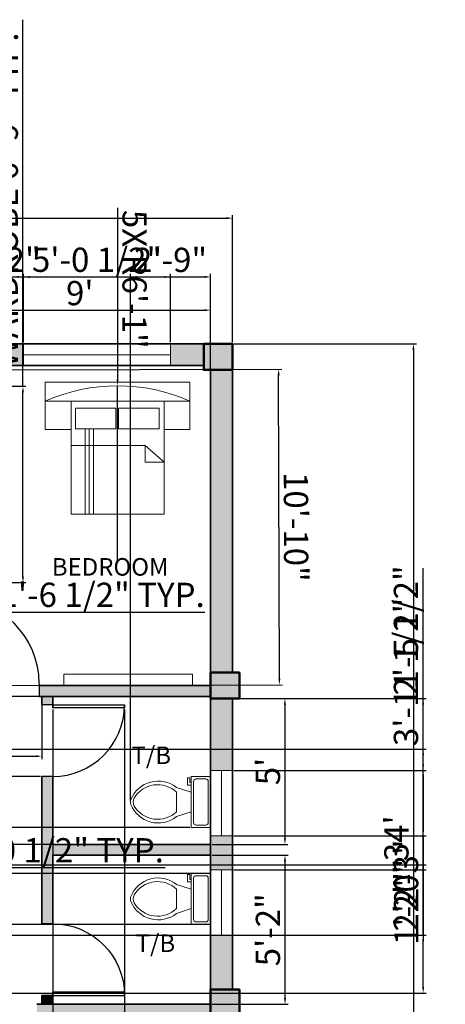
# Model space of a CAD drawing. Units: inches. Extents: x 2312 to 2808, y 1290 to 1909.
# Tile 5 of 5: x 2633 to 2808, y 1503 to 1909. Entities that reach past the tile are written whole.
import ezdxf

# ---------------------------------------------------------------- set-up
doc = ezdxf.new("R2010")
doc.units = ezdxf.units.IN
for name, color, linetype, lineweight in [('A-ANNO-DIMS', 2, 'Continuous', 18), ('A-AREA-IDEN', 7, 'Continuous', 25), ('A-COLS-PATT', 1, 'Continuous', 13), ('A-FLOR-CASE', 181, 'Continuous', 20), ('A-FLOR-FIXT', 9, 'Continuous', 18), ('A-WALL-PATT', 150, 'Continuous', 13), ('COLUMN', 1, 'Continuous', 50), ('DOOR', 50, 'Continuous', 25), ('FUR', 130, 'Continuous', 18), ('WALL', 7, 'Continuous', 35), ('WINDOW', 70, 'Continuous', 18)]:
    doc.layers.add(name, color=color, linetype=linetype, lineweight=lineweight)
doc.styles.get("Standard").update_dxf_attribs({"font": 'arial.ttf'})
doc.dimstyles.new('ISO-25', dxfattribs={"dimtxt": 10, "dimasz": 2.5, "dimexe": 1.25, "dimexo": 0.625, "dimtad": 1, "dimdec": 0, "dimlunit": 4, "dimtxsty": 'Standard', "dimcen": 2.5, "dimadec": 0, "dimazin": 0, "dimtfac": 1, "dimtdec": 0, "dimtmove": 0, "dimatfit": 3, "dimfxl": 1, "dimarcsym": 0})

# ---------------------------------------------------------------- blocks, each defined once
blk = doc.blocks.new('*U2')
for p, q in [((0, 0), (0, -6)), ((40, 0), (40, -6))]:
    blk.add_line(p, q)
blk.add_lwpolyline([(0, 0), (0, 40), (1.75, 40), (1.75, 0)], close=True)
blk.add_arc((0, 0), 40, 0, 90)
blk = doc.blocks.new('*U4')
for p, q in [((9.5, -6), (9.5, -2)), ((-8, -8.5), (-8, -8)), ((-7, -8), (-7, -9.5)), ((-4, -8), (-6, -14)), ((4, -8), (6, -14)), ((-10, -8.5), (-8, -8.5)), ((-10, -9.5), (-10, -8.5)), ((-7, -9.5), (-10, -9.5)), ((4, -14), (-4, -14))]:
    blk.add_line(p, q)
blk.add_lwpolyline([(10.5, -8), (10.5, 0), (-10.5, 0), (-10.5, -8)], close=True)
for points in [[(-9.5, -2), (-9.5, -6)], [(8.5, -1), (-8.5, -1)], [(-8.5, -7), (8.5, -7)]]:
    blk.add_lwpolyline(points)
for centre, radius, start, end in [((-8.62, -1.88), 0.884, 81.8699, 188.1301), ((8.62, -1.88), 0.884, 351.8699, 98.1301), ((-8.62, -6.12), 0.884, 171.8699, 278.1301), ((8.62, -6.12), 0.884, 261.8699, 8.1301), ((3.52, -21.58), 12.17, 141.4691, 247.9714), ((4.2, -21.82), 11.33, 136.3677, 238.9468), ((-3.52, -21.58), 12.17, 292.0284, 38.5307), ((-4.2, -21.82), 11.33, 301.053, 43.6321), ((0, -27.88), 4, 245.7318, 294.2682), ((0, -29), 4, 254.8605, 285.1395)]:
    blk.add_arc(centre, radius, start, end)
blk = doc.blocks.new('*D5')
at = {"layer": 'A-ANNO-DIMS', "color": 0, "lineweight": -2, "transparency": 16777216}
for p, q in [((2360.43, 1776.34), (2360.43, 1828.83)), ((2720.43, 1776.34), (2720.43, 1828.83)), ((2362.93, 1827.58), (2717.93, 1827.58))]:
    blk.add_line(p, q, dxfattribs=at)
at = {"layer": 'A-ANNO-DIMS', "color": 0, "transparency": 16777216}
for points in [[(2362.93, 1828), (2362.93, 1827.17), (2360.43, 1827.58)], [(2717.93, 1828), (2717.93, 1827.17), (2720.43, 1827.58)]]:
    blk.add_solid(points, dxfattribs=at)
at = {"layer": 'Defpoints', "color": 0, "transparency": 16777216}
for p in [(2720.43, 1827.58), (2360.43, 1775.72), (2720.43, 1775.72)]:
    blk.add_point(p, dxfattribs=at)
at = {"layer": 'A-ANNO-DIMS', "color": 0, "transparency": 16777216, "insert": (2540.43, 1833.32), "char_height": 10, "attachment_point": 5}
blk.add_mtext("30'", dxfattribs=at)
blk = doc.blocks.new('*D6')
at = {"layer": 'A-ANNO-DIMS', "color": 0, "lineweight": -2, "transparency": 16777216}
for p, q in [((2721.06, 1775.72), (2796.28, 1775.72)), ((2795.03, 1773.22), (2795.03, 1370.22)), ((2721.06, 1367.72), (2796.28, 1367.72))]:
    blk.add_line(p, q, dxfattribs=at)
at = {"layer": 'A-ANNO-DIMS', "color": 0, "transparency": 16777216}
for points in [[(2794.62, 1773.22), (2795.45, 1773.22), (2795.03, 1775.72)], [(2794.62, 1370.22), (2795.45, 1370.22), (2795.03, 1367.72)]]:
    blk.add_solid(points, dxfattribs=at)
at = {"layer": 'Defpoints', "color": 0, "transparency": 16777216}
for p in [(2720.43, 1775.72), (2720.43, 1367.72), (2795.03, 1367.72)]:
    blk.add_point(p, dxfattribs=at)
at = {"layer": 'A-ANNO-DIMS', "color": 0, "transparency": 16777216, "insert": (2789.3, 1571.72), "char_height": 10, "attachment_point": 5, "rotation": 90}
blk.add_mtext("34'", dxfattribs=at)
blk = doc.blocks.new('*D11')
at = {"layer": 'A-ANNO-DIMS', "color": 0, "lineweight": -2, "transparency": 16777216}
for p, q in [((2603.61, 1765.57), (2603.61, 1790.88)), ((2606.11, 1789.63), (2708.93, 1789.63)), ((2711.43, 1765.57), (2711.43, 1790.88))]:
    blk.add_line(p, q, dxfattribs=at)
at = {"layer": 'A-ANNO-DIMS', "color": 0, "transparency": 16777216}
for points in [[(2606.11, 1790.04), (2606.11, 1789.21), (2603.61, 1789.63)], [(2708.93, 1790.04), (2708.93, 1789.21), (2711.43, 1789.63)]]:
    blk.add_solid(points, dxfattribs=at)
at = {"layer": 'Defpoints', "color": 0, "transparency": 16777216}
for p in [(2711.43, 1789.63), (2603.61, 1764.94), (2711.43, 1764.94)]:
    blk.add_point(p, dxfattribs=at)
at = {"layer": 'A-ANNO-DIMS', "color": 0, "transparency": 16777216, "insert": (2657.52, 1795.36), "char_height": 10, "attachment_point": 5}
blk.add_mtext("9'", dxfattribs=at)
blk = doc.blocks.new('*D12')
at = {"layer": 'A-ANNO-DIMS', "color": 0, "lineweight": -2, "transparency": 16777216}
for p, q in [((2604.24, 1764.94), (2740.72, 1765.28)), ((2739.79, 1637.55), (2739.48, 1762.78)), ((2604.56, 1634.72), (2741.04, 1635.06))]:
    blk.add_line(p, q, dxfattribs=at)
at = {"layer": 'A-ANNO-DIMS', "color": 0, "transparency": 16777216}
for points in [[(2739.89, 1762.78), (2739.06, 1762.78), (2739.47, 1765.28)], [(2740.2, 1637.56), (2739.37, 1637.55), (2739.79, 1635.05)]]:
    blk.add_solid(points, dxfattribs=at)
at = {"layer": 'Defpoints', "color": 0, "transparency": 16777216}
for p in [(2603.61, 1764.94), (2739.47, 1765.28), (2603.93, 1634.72)]:
    blk.add_point(p, dxfattribs=at)
at = {"layer": 'A-ANNO-DIMS', "color": 0, "transparency": 16777216, "insert": (2745.36, 1700.18), "char_height": 10, "attachment_point": 5, "rotation": 270.1423}
blk.add_mtext('10\'-10"', dxfattribs=at)
blk = doc.blocks.new('*D13')
at = {"layer": 'A-ANNO-DIMS', "color": 0, "lineweight": -2, "transparency": 16777216}
for p, q in [((2712.06, 1629.34), (2743.32, 1629.34)), ((2742.07, 1626.84), (2742.07, 1571.72)), ((2712.06, 1569.22), (2743.32, 1569.22))]:
    blk.add_line(p, q, dxfattribs=at)
at = {"layer": 'A-ANNO-DIMS', "color": 0, "transparency": 16777216}
for points in [[(2741.66, 1626.84), (2742.49, 1626.84), (2742.07, 1629.34)], [(2741.66, 1571.72), (2742.49, 1571.72), (2742.07, 1569.22)]]:
    blk.add_solid(points, dxfattribs=at)
at = {"layer": 'Defpoints', "color": 0, "transparency": 16777216}
for p in [(2711.43, 1629.34), (2711.43, 1569.22), (2742.07, 1569.22)]:
    blk.add_point(p, dxfattribs=at)
at = {"layer": 'A-ANNO-DIMS', "color": 0, "transparency": 16777216, "insert": (2736.36, 1599.28), "char_height": 10, "attachment_point": 5, "rotation": 90}
blk.add_mtext("5'", dxfattribs=at)
blk = doc.blocks.new('*D14')
at = {"layer": 'A-ANNO-DIMS', "color": 0, "lineweight": -2, "transparency": 16777216}
for p, q in [((2712.06, 1564.72), (2743.34, 1564.72)), ((2742.09, 1562.22), (2742.09, 1505.72)), ((2712.06, 1503.22), (2743.34, 1503.22))]:
    blk.add_line(p, q, dxfattribs=at)
at = {"layer": 'A-ANNO-DIMS', "color": 0, "transparency": 16777216}
for points in [[(2741.67, 1562.22), (2742.5, 1562.22), (2742.09, 1564.72)], [(2741.67, 1505.72), (2742.5, 1505.72), (2742.09, 1503.22)]]:
    blk.add_solid(points, dxfattribs=at)
at = {"layer": 'Defpoints', "color": 0, "transparency": 16777216}
for p in [(2711.43, 1564.72), (2711.43, 1503.22), (2742.09, 1503.22)]:
    blk.add_point(p, dxfattribs=at)
at = {"layer": 'A-ANNO-DIMS', "color": 0, "transparency": 16777216, "insert": (2736.35, 1533.97), "char_height": 10, "attachment_point": 5, "rotation": 90}
blk.add_mtext('5\'-2"', dxfattribs=at)
blk = doc.blocks.new('*D22')
at = {"layer": 'A-ANNO-DIMS', "color": 0, "lineweight": -2, "transparency": 16777216}
for p, q in [((2486.93, 1629.59), (2486.93, 1604.33)), ((2641.91, 1629.59), (2641.91, 1604.33)), ((2489.43, 1605.58), (2639.41, 1605.58))]:
    blk.add_line(p, q, dxfattribs=at)
at = {"layer": 'A-ANNO-DIMS', "color": 0, "transparency": 16777216}
for points in [[(2489.43, 1606), (2489.43, 1605.17), (2486.93, 1605.58)], [(2639.41, 1606), (2639.41, 1605.17), (2641.91, 1605.58)]]:
    blk.add_solid(points, dxfattribs=at)
at = {"layer": 'Defpoints', "color": 0, "transparency": 16777216}
for p in [(2486.93, 1630.22), (2641.91, 1630.22), (2641.91, 1605.58)]:
    blk.add_point(p, dxfattribs=at)
at = {"layer": 'A-ANNO-DIMS', "color": 0, "transparency": 16777216, "insert": (2564.42, 1611.23), "char_height": 10, "attachment_point": 5}
blk.add_mtext('12\'-11"', dxfattribs=at)
blk = doc.blocks.new('BED-DOUBLE')
for p, q in [((0, 46.6), (0, 54.42)), ((0, 54.42), (59.67, 54.42)), ((59.67, 54.42), (59.67, 46.6)), ((16.43, 35.15), (16.43, 0)), ((18.15, 35.15), (18.15, 0)), ((19.9, 35.15), (19.9, 0)), ((10.68, 28.37), (10.68, 28.37)), ((10.68, 28.37), (41.23, 28.37)), ((41.23, 28.37), (41.23, 21.43)), ((48.99, 21.43), (41.23, 28.37)), ((41.23, 21.43), (48.99, 21.43))]:
    blk.add_line(p, q)
for points in [[(10.68, 46.6), (0, 46.6), (0, 34.89), (10.68, 34.89)], [(10.68, 46.6), (48.99, 46.6), (48.99, 0), (10.68, 0)], [(59.67, 46.6), (48.99, 46.6), (48.99, 34.89), (59.67, 34.89)], [(12.51, 43.74), (29.18, 43.74), (29.18, 35.15), (12.51, 35.15)], [(30.28, 43.78), (46.95, 43.78), (46.95, 35.19), (30.28, 35.19)]]:
    blk.add_lwpolyline(points, close=True)
blk.add_arc((29.84, -20.26), 73.22, 65.9516, 114.0484)
blk = doc.blocks.new('BEDROOM-WALL-UNIT')
blk.add_lwpolyline([(0, 0), (52.94, 0), (52.94, 4.76), (0, 4.76)], close=True)
blk = doc.blocks.new('*D31')
at = {"layer": 'A-ANNO-DIMS', "color": 0, "lineweight": -2, "transparency": 16777216}
for p, q in [((2634.1, 1758.19), (2634.1, 1909.46)), ((2622.58, 1758.19), (2635.35, 1758.19)), ((2634.1, 1679.72), (2634.1, 1755.69)), ((2622.58, 1677.22), (2635.35, 1677.22))]:
    blk.add_line(p, q, dxfattribs=at)
at = {"layer": 'A-ANNO-DIMS', "color": 0, "transparency": 16777216}
for points in [[(2633.68, 1755.69), (2634.51, 1755.69), (2634.1, 1758.19)], [(2633.68, 1679.72), (2634.51, 1679.72), (2634.1, 1677.22)]]:
    blk.add_solid(points, dxfattribs=at)
at = {"layer": 'Defpoints', "color": 0, "transparency": 16777216}
for p in [(2621.95, 1758.19), (2634.1, 1758.19), (2621.95, 1677.22)]:
    blk.add_point(p, dxfattribs=at)
at = {"layer": 'A-ANNO-DIMS', "color": 0, "transparency": 16777216, "insert": (2628.3, 1835.07), "char_height": 10, "attachment_point": 5, "rotation": 90}
blk.add_mtext('WARDROBE 6\'-9" TYP.', dxfattribs=at)
blk = doc.blocks.new('*D32')
at = {"layer": 'A-ANNO-DIMS', "color": 0, "lineweight": -2, "transparency": 16777216}
for p, q in [((2603.61, 1676.59), (2603.61, 1663.82)), ((2621.95, 1676.59), (2621.95, 1663.82)), ((2606.11, 1665.07), (2619.45, 1665.07)), ((2621.95, 1665.07), (2709.02, 1665.07))]:
    blk.add_line(p, q, dxfattribs=at)
at = {"layer": 'A-ANNO-DIMS', "color": 0, "transparency": 16777216}
for points in [[(2606.11, 1665.49), (2606.11, 1664.65), (2603.61, 1665.07)], [(2619.45, 1665.49), (2619.45, 1664.65), (2621.95, 1665.07)]]:
    blk.add_solid(points, dxfattribs=at)
at = {"layer": 'Defpoints', "color": 0, "transparency": 16777216}
for p in [(2603.61, 1677.22), (2621.95, 1677.22), (2621.95, 1665.07)]:
    blk.add_point(p, dxfattribs=at)
at = {"layer": 'A-ANNO-DIMS', "color": 0, "transparency": 16777216, "insert": (2666.73, 1670.87), "char_height": 10, "attachment_point": 5}
blk.add_mtext('1\'-6 1/2" TYP.', dxfattribs=at)
blk = doc.blocks.new('*D36')
at = {"layer": 'A-ANNO-DIMS', "color": 0, "lineweight": -2, "transparency": 16777216}
for p, q in [((2586.49, 1560.99), (2586.49, 1558.44)), ((2596.99, 1560.99), (2596.99, 1558.44)), ((2588.99, 1559.69), (2594.49, 1559.69)), ((2596.99, 1559.69), (2692.76, 1559.69))]:
    blk.add_line(p, q, dxfattribs=at)
at = {"layer": 'A-ANNO-DIMS', "color": 0, "transparency": 16777216}
for points in [[(2588.99, 1560.1), (2588.99, 1559.27), (2586.49, 1559.69)], [(2594.49, 1560.1), (2594.49, 1559.27), (2596.99, 1559.69)]]:
    blk.add_solid(points, dxfattribs=at)
at = {"layer": 'Defpoints', "color": 0, "transparency": 16777216}
for p in [(2586.49, 1561.62), (2596.99, 1561.62), (2596.99, 1559.69)]:
    blk.add_point(p, dxfattribs=at)
at = {"layer": 'A-ANNO-DIMS', "color": 0, "transparency": 16777216, "insert": (2646.12, 1565.48), "char_height": 10, "attachment_point": 5}
blk.add_mtext('0\'-10 1/2" TYP.', dxfattribs=at)
blk = doc.blocks.new('*D39')
at = {"layer": 'A-ANNO-DIMS', "color": 0, "lineweight": -2, "transparency": 16777216}
for p, q in [((2646.41, 1564.09), (2646.41, 1326.46)), ((2711.43, 1564.09), (2711.43, 1326.46)), ((2648.91, 1327.71), (2708.93, 1327.71))]:
    blk.add_line(p, q, dxfattribs=at)
at = {"layer": 'A-ANNO-DIMS', "color": 0, "transparency": 16777216}
for points in [[(2648.91, 1328.13), (2648.91, 1327.3), (2646.41, 1327.71)], [(2708.93, 1328.13), (2708.93, 1327.3), (2711.43, 1327.71)]]:
    blk.add_solid(points, dxfattribs=at)
at = {"layer": 'Defpoints', "color": 0, "transparency": 16777216}
for p in [(2646.41, 1564.72), (2711.43, 1564.72), (2711.43, 1327.71)]:
    blk.add_point(p, dxfattribs=at)
at = {"layer": 'A-ANNO-DIMS', "color": 0, "transparency": 16777216, "insert": (2678.92, 1333.42), "char_height": 10, "attachment_point": 5}
blk.add_mtext('5\'-5"', dxfattribs=at)
blk = doc.blocks.new('*D48')
at = {"layer": 'A-ANNO-DIMS', "color": 0, "lineweight": -2, "transparency": 16777216}
for p, q in [((2571.02, 1776.34), (2571.02, 1804.57)), ((2634.31, 1776.34), (2634.31, 1804.57)), ((2573.52, 1803.32), (2631.81, 1803.32))]:
    blk.add_line(p, q, dxfattribs=at)
at = {"layer": 'A-ANNO-DIMS', "color": 0, "transparency": 16777216}
for points in [[(2573.52, 1803.73), (2573.52, 1802.9), (2571.02, 1803.32)], [(2631.81, 1803.73), (2631.81, 1802.9), (2634.31, 1803.32)]]:
    blk.add_solid(points, dxfattribs=at)
at = {"layer": 'Defpoints', "color": 0, "transparency": 16777216}
for p in [(2634.31, 1803.32), (2571.02, 1775.72), (2634.31, 1775.72)]:
    blk.add_point(p, dxfattribs=at)
at = {"layer": 'A-ANNO-DIMS', "color": 0, "transparency": 16777216, "insert": (2602.66, 1809.12), "char_height": 10, "attachment_point": 5}
blk.add_mtext('5\'-3 1/2"', dxfattribs=at)
blk = doc.blocks.new('*D49')
at = {"layer": 'A-ANNO-DIMS', "color": 0, "lineweight": -2, "transparency": 16777216}
for p, q in [((2634.31, 1776.34), (2634.31, 1804.57)), ((2694.96, 1776.34), (2694.96, 1804.57)), ((2636.81, 1803.32), (2692.46, 1803.32))]:
    blk.add_line(p, q, dxfattribs=at)
at = {"layer": 'A-ANNO-DIMS', "color": 0, "transparency": 16777216}
for points in [[(2636.81, 1803.73), (2636.81, 1802.9), (2634.31, 1803.32)], [(2692.46, 1803.73), (2692.46, 1802.9), (2694.96, 1803.32)]]:
    blk.add_solid(points, dxfattribs=at)
at = {"layer": 'Defpoints', "color": 0, "transparency": 16777216}
for p in [(2694.96, 1803.32), (2634.31, 1775.72), (2694.96, 1775.72)]:
    blk.add_point(p, dxfattribs=at)
at = {"layer": 'A-ANNO-DIMS', "color": 0, "transparency": 16777216, "insert": (2664.64, 1809.11), "char_height": 10, "attachment_point": 5}
blk.add_mtext('5\'-0 1/2"', dxfattribs=at)
blk = doc.blocks.new('*D51')
at = {"layer": 'A-ANNO-DIMS', "color": 0, "lineweight": -2, "transparency": 16777216}
for p, q in [((2646.41, 1624.89), (2646.41, 1326.46)), ((2675.95, 1624.89), (2675.95, 1326.46)), ((2648.91, 1327.71), (2673.45, 1327.71)), ((2675.95, 1327.71), (2729.75, 1327.71))]:
    blk.add_line(p, q, dxfattribs=at)
at = {"layer": 'A-ANNO-DIMS', "color": 0, "transparency": 16777216}
for points in [[(2648.91, 1328.13), (2648.91, 1327.3), (2646.41, 1327.71)], [(2673.45, 1328.13), (2673.45, 1327.3), (2675.95, 1327.71)]]:
    blk.add_solid(points, dxfattribs=at)
at = {"layer": 'Defpoints', "color": 0, "transparency": 16777216}
for p in [(2646.41, 1625.52), (2675.95, 1625.52), (2675.95, 1327.71)]:
    blk.add_point(p, dxfattribs=at)
at = {"layer": 'A-ANNO-DIMS', "color": 0, "transparency": 16777216, "insert": (2704.1, 1333.51), "char_height": 10, "attachment_point": 5}
blk.add_mtext('2\'-5 1/2"', dxfattribs=at)
blk = doc.blocks.new('*D54')
at = {"layer": 'A-ANNO-DIMS', "color": 0, "lineweight": -2, "transparency": 16777216}
for p, q in [((2545.01, 1581.25), (2545.01, 1804.57)), ((2586.49, 1581.25), (2586.49, 1804.57)), ((2547.51, 1803.32), (2583.99, 1803.32)), ((2586.49, 1803.32), (2640.12, 1803.32))]:
    blk.add_line(p, q, dxfattribs=at)
at = {"layer": 'A-ANNO-DIMS', "color": 0, "transparency": 16777216}
for points in [[(2547.51, 1803.73), (2547.51, 1802.9), (2545.01, 1803.32)], [(2583.99, 1803.73), (2583.99, 1802.9), (2586.49, 1803.32)]]:
    blk.add_solid(points, dxfattribs=at)
at = {"layer": 'Defpoints', "color": 0, "transparency": 16777216}
for p in [(2586.49, 1803.32), (2545.01, 1580.62), (2586.49, 1580.62)]:
    blk.add_point(p, dxfattribs=at)
at = {"layer": 'A-ANNO-DIMS', "color": 0, "transparency": 16777216, "insert": (2614.56, 1809.12), "char_height": 10, "attachment_point": 5}
blk.add_mtext('3\'-5 1/2"', dxfattribs=at)
blk = doc.blocks.new('*D56')
at = {"layer": 'A-ANNO-DIMS', "color": 0, "lineweight": -2, "transparency": 16777216}
for p, q in [((2721.06, 1599.72), (2800.28, 1599.72)), ((2799.03, 1597.22), (2799.03, 1575.18)), ((2721.06, 1572.68), (2800.28, 1572.68)), ((2799.03, 1572.68), (2799.03, 1542.18))]:
    blk.add_line(p, q, dxfattribs=at)
at = {"layer": 'A-ANNO-DIMS', "color": 0, "transparency": 16777216}
for points in [[(2798.62, 1597.22), (2799.45, 1597.22), (2799.03, 1599.72)], [(2798.62, 1575.18), (2799.45, 1575.18), (2799.03, 1572.68)]]:
    blk.add_solid(points, dxfattribs=at)
at = {"layer": 'Defpoints', "color": 0, "transparency": 16777216}
for p in [(2720.43, 1599.72), (2720.43, 1572.68), (2799.03, 1572.68)]:
    blk.add_point(p, dxfattribs=at)
at = {"layer": 'A-ANNO-DIMS', "color": 0, "transparency": 16777216, "insert": (2793.3, 1556.18), "char_height": 10, "attachment_point": 5, "rotation": 90}
blk.add_mtext('2\'-3"', dxfattribs=at)
blk = doc.blocks.new('*D57')
at = {"layer": 'A-ANNO-DIMS', "color": 0, "lineweight": -2, "transparency": 16777216}
for p, q in [((2721.06, 1572.68), (2800.28, 1572.68)), ((2799.03, 1570.18), (2799.03, 1561.21)), ((2721.06, 1558.71), (2800.28, 1558.71)), ((2799.03, 1558.71), (2799.03, 1529.32))]:
    blk.add_line(p, q, dxfattribs=at)
at = {"layer": 'A-ANNO-DIMS', "color": 0, "transparency": 16777216}
for points in [[(2798.62, 1570.18), (2799.45, 1570.18), (2799.03, 1572.68)], [(2798.62, 1561.21), (2799.45, 1561.21), (2799.03, 1558.71)]]:
    blk.add_solid(points, dxfattribs=at)
at = {"layer": 'Defpoints', "color": 0, "transparency": 16777216}
for p in [(2720.43, 1572.68), (2720.43, 1558.71), (2799.03, 1558.71)]:
    blk.add_point(p, dxfattribs=at)
at = {"layer": 'A-ANNO-DIMS', "color": 0, "transparency": 16777216, "insert": (2793.39, 1542.76), "char_height": 10, "attachment_point": 5, "rotation": 90}
blk.add_mtext('1\'-2"', dxfattribs=at)
blk = doc.blocks.new('*D58')
at = {"layer": 'A-ANNO-DIMS', "color": 0, "lineweight": -2, "transparency": 16777216}
for p, q in [((2799.03, 1629.34), (2799.03, 1683.14)), ((2721.06, 1629.34), (2800.28, 1629.34)), ((2799.03, 1602.22), (2799.03, 1626.84)), ((2721.06, 1599.72), (2800.28, 1599.72))]:
    blk.add_line(p, q, dxfattribs=at)
at = {"layer": 'A-ANNO-DIMS', "color": 0, "transparency": 16777216}
for points in [[(2798.62, 1626.84), (2799.45, 1626.84), (2799.03, 1629.34)], [(2798.62, 1602.22), (2799.45, 1602.22), (2799.03, 1599.72)]]:
    blk.add_solid(points, dxfattribs=at)
at = {"layer": 'Defpoints', "color": 0, "transparency": 16777216}
for p in [(2720.43, 1629.34), (2799.03, 1629.34), (2720.43, 1599.72)]:
    blk.add_point(p, dxfattribs=at)
at = {"layer": 'A-ANNO-DIMS', "color": 0, "transparency": 16777216, "insert": (2793.24, 1657.49), "char_height": 10, "attachment_point": 5, "rotation": 90}
blk.add_mtext('2\'-5 1/2"', dxfattribs=at)
blk = doc.blocks.new('*D63')
at = {"layer": 'A-ANNO-DIMS', "color": 0, "lineweight": -2, "transparency": 16777216}
for p, q in [((2799.03, 1531.79), (2799.03, 1562.3)), ((2433.46, 1531.79), (2800.28, 1531.79)), ((2799.03, 1510.3), (2799.03, 1529.29)), ((2433.46, 1507.8), (2800.28, 1507.8))]:
    blk.add_line(p, q, dxfattribs=at)
at = {"layer": 'A-ANNO-DIMS', "color": 0, "transparency": 16777216}
for points in [[(2798.62, 1529.29), (2799.45, 1529.29), (2799.03, 1531.79)], [(2798.62, 1510.3), (2799.45, 1510.3), (2799.03, 1507.8)]]:
    blk.add_solid(points, dxfattribs=at)
at = {"layer": 'Defpoints', "color": 0, "transparency": 16777216}
for p in [(2432.83, 1531.79), (2799.03, 1531.79), (2432.83, 1507.8)]:
    blk.add_point(p, dxfattribs=at)
at = {"layer": 'A-ANNO-DIMS', "color": 0, "transparency": 16777216, "insert": (2793.3, 1548.3), "char_height": 10, "attachment_point": 5, "rotation": 90}
blk.add_mtext('2\'-0"', dxfattribs=at)
blk = doc.blocks.new('*D64')
at = {"layer": 'A-ANNO-DIMS', "color": 0, "lineweight": -2, "transparency": 16777216}
for p, q in [((2678.43, 1587.31), (2678.43, 1804.57)), ((2711.43, 1597.81), (2711.43, 1804.57)), ((2680.93, 1803.32), (2708.93, 1803.32))]:
    blk.add_line(p, q, dxfattribs=at)
at = {"layer": 'A-ANNO-DIMS', "color": 0, "transparency": 16777216}
for points in [[(2680.93, 1803.73), (2680.93, 1802.9), (2678.43, 1803.32)], [(2708.93, 1803.73), (2708.93, 1802.9), (2711.43, 1803.32)]]:
    blk.add_solid(points, dxfattribs=at)
at = {"layer": 'Defpoints', "color": 0, "transparency": 16777216}
for p in [(2711.43, 1803.32), (2711.43, 1597.18), (2678.43, 1586.68)]:
    blk.add_point(p, dxfattribs=at)
at = {"layer": 'A-ANNO-DIMS', "color": 0, "transparency": 16777216, "insert": (2694.93, 1809.05), "char_height": 10, "attachment_point": 5}
blk.add_mtext('2\'-9"', dxfattribs=at)
blk = doc.blocks.new('*D65')
at = {"layer": 'A-ANNO-DIMS', "color": 0, "lineweight": -2, "transparency": 16777216}
for p, q in [((2710.81, 1557.21), (2331.58, 1557.21)), ((2332.83, 1554.71), (2332.83, 1538.71)), ((2710.81, 1536.21), (2331.58, 1536.21)), ((2332.83, 1536.21), (2332.83, 1506.82))]:
    blk.add_line(p, q, dxfattribs=at)
at = {"layer": 'A-ANNO-DIMS', "color": 0, "transparency": 16777216}
for points in [[(2332.42, 1554.71), (2333.25, 1554.71), (2332.83, 1557.21)], [(2332.42, 1538.71), (2333.25, 1538.71), (2332.83, 1536.21)]]:
    blk.add_solid(points, dxfattribs=at)
at = {"layer": 'Defpoints', "color": 0, "transparency": 16777216}
for p in [(2711.43, 1557.21), (2332.83, 1536.21), (2711.43, 1536.21)]:
    blk.add_point(p, dxfattribs=at)
at = {"layer": 'A-ANNO-DIMS', "color": 0, "transparency": 16777216, "insert": (2327.1, 1520.27), "char_height": 10, "attachment_point": 5, "rotation": 90}
blk.add_mtext('1\'-9"', dxfattribs=at)
blk = doc.blocks.new('*D71')
at = {"layer": 'A-ANNO-DIMS', "color": 0, "lineweight": -2, "transparency": 16777216}
for p, q in [((2587.32, 1629.59), (2587.32, 1326.46)), ((2603.93, 1629.59), (2603.93, 1326.46)), ((2589.82, 1327.71), (2601.43, 1327.71)), ((2603.93, 1327.71), (2656.63, 1327.71))]:
    blk.add_line(p, q, dxfattribs=at)
at = {"layer": 'A-ANNO-DIMS', "color": 0, "transparency": 16777216}
for points in [[(2589.82, 1328.13), (2589.82, 1327.3), (2587.32, 1327.71)], [(2601.43, 1328.13), (2601.43, 1327.3), (2603.93, 1327.71)]]:
    blk.add_solid(points, dxfattribs=at)
at = {"layer": 'Defpoints', "color": 0, "transparency": 16777216}
for p in [(2587.32, 1630.22), (2603.93, 1630.22), (2603.93, 1327.71)]:
    blk.add_point(p, dxfattribs=at)
at = {"layer": 'A-ANNO-DIMS', "color": 0, "transparency": 16777216, "insert": (2631.53, 1333.51), "char_height": 10, "attachment_point": 5}
blk.add_mtext('1\'-4 1/2"', dxfattribs=at)
blk = doc.blocks.new('*D72')
at = {"layer": 'A-ANNO-DIMS', "color": 0, "lineweight": -2, "transparency": 16777216}
for p, q in [((2702.81, 1576.18), (2331.58, 1576.18)), ((2332.83, 1573.68), (2332.83, 1571.72)), ((2710.81, 1569.22), (2331.58, 1569.22)), ((2332.83, 1569.22), (2332.83, 1538.88))]:
    blk.add_line(p, q, dxfattribs=at)
at = {"layer": 'A-ANNO-DIMS', "color": 0, "transparency": 16777216}
for points in [[(2332.42, 1573.68), (2333.25, 1573.68), (2332.83, 1576.18)], [(2332.42, 1571.72), (2333.25, 1571.72), (2332.83, 1569.22)]]:
    blk.add_solid(points, dxfattribs=at)
at = {"layer": 'Defpoints', "color": 0, "transparency": 16777216}
for p in [(2703.43, 1576.18), (2332.83, 1569.22), (2711.43, 1569.22)]:
    blk.add_point(p, dxfattribs=at)
at = {"layer": 'A-ANNO-DIMS', "color": 0, "transparency": 16777216, "insert": (2327.1, 1552.8), "char_height": 10, "attachment_point": 5, "rotation": 90}
blk.add_mtext('0\'-7"', dxfattribs=at)
blk = doc.blocks.new('*D74')
at = {"layer": 'A-ANNO-DIMS', "color": 0, "lineweight": -2, "transparency": 16777216}
for p, q in [((2799.03, 1608.44), (2799.03, 1669.84)), ((2403.21, 1608.44), (2800.28, 1608.44)), ((2799.03, 1563.31), (2799.03, 1605.94)), ((2403.21, 1560.81), (2800.28, 1560.81))]:
    blk.add_line(p, q, dxfattribs=at)
at = {"layer": 'A-ANNO-DIMS', "color": 0, "transparency": 16777216}
for points in [[(2798.62, 1605.94), (2799.45, 1605.94), (2799.03, 1608.44)], [(2798.62, 1563.31), (2799.45, 1563.31), (2799.03, 1560.81)]]:
    blk.add_solid(points, dxfattribs=at)
at = {"layer": 'Defpoints', "color": 0, "transparency": 16777216}
for p in [(2402.58, 1608.44), (2799.03, 1608.44), (2402.58, 1560.81)]:
    blk.add_point(p, dxfattribs=at)
at = {"layer": 'A-ANNO-DIMS', "color": 0, "transparency": 16777216, "insert": (2793.24, 1640.39), "char_height": 10, "attachment_point": 5, "rotation": 90}
blk.add_mtext('3\'-11 1/2"', dxfattribs=at)
blk = doc.blocks.new('*D75')
at = {"layer": 'A-ANNO-DIMS', "color": 0, "lineweight": -2, "transparency": 16777216}
for p, q in [((2641.28, 1630.22), (2331.58, 1630.22)), ((2332.83, 1627.72), (2332.83, 1599.71)), ((2641.28, 1597.21), (2331.58, 1597.21))]:
    blk.add_line(p, q, dxfattribs=at)
at = {"layer": 'A-ANNO-DIMS', "color": 0, "transparency": 16777216}
for points in [[(2332.42, 1627.72), (2333.25, 1627.72), (2332.83, 1630.22)], [(2332.42, 1599.71), (2333.25, 1599.71), (2332.83, 1597.21)]]:
    blk.add_solid(points, dxfattribs=at)
at = {"layer": 'Defpoints', "color": 0, "transparency": 16777216}
for p in [(2641.91, 1630.22), (2332.83, 1597.21), (2641.91, 1597.21)]:
    blk.add_point(p, dxfattribs=at)
at = {"layer": 'A-ANNO-DIMS', "color": 0, "transparency": 16777216, "insert": (2327.1, 1613.71), "char_height": 10, "attachment_point": 5, "rotation": 90}
blk.add_mtext('2\'-9"', dxfattribs=at)
blk = doc.blocks.new('*D78')
at = {"layer": 'A-ANNO-DIMS', "color": 0, "lineweight": -2, "transparency": 16777216}
for p, q in [((2673.09, 1831.79), (2673.09, 1760.92)), ((2673.09, 1685.2), (2673.09, 1758.42))]:
    blk.add_line(p, q, dxfattribs=at)
at = {"layer": 'A-ANNO-DIMS', "color": 0, "transparency": 16777216}
blk.add_solid([(2673.51, 1760.92), (2672.68, 1760.92), (2673.09, 1758.42)], dxfattribs=at)
at = {"layer": 'Defpoints', "color": 0, "transparency": 16777216}
for p in [(2673.09, 1758.42), (2673.09, 1685.2)]:
    blk.add_point(p, dxfattribs=at)
at = {"layer": 'A-ANNO-DIMS', "color": 0, "transparency": 16777216, "insert": (2678.82, 1802.35), "char_height": 10, "attachment_point": 5, "rotation": 270.0002}
blk.add_mtext('5X R6\'-1"', dxfattribs=at)

msp = doc.modelspace()

# ---------------------------------------------------------------- hatches: boundary and pattern name
at = {"layer": 'A-COLS-PATT'}
h = msp.add_hatch(color=256, dxfattribs=at)
h.dxf.hatch_style = 1
h.paths.add_polyline_path([(2372.28, 1775.72), (2360.43, 1775.72), (2360.43, 1764.94), (2372.28, 1764.94)])
h.paths.add_polyline_path([(2486.97, 1775.72), (2475.12, 1775.72), (2475.12, 1764.94), (2486.93, 1764.94), (2486.93, 1766.72)])
h.paths.add_polyline_path([(2610.92, 1775.72), (2599.07, 1775.72), (2599.07, 1766.72), (2599.11, 1766.72), (2599.11, 1764.94), (2610.92, 1764.94)])
h.paths.add_polyline_path([(2720.43, 1775.72), (2708.59, 1775.72), (2708.59, 1764.94), (2720.43, 1764.94)])
h.paths.add_polyline_path([(2723.28, 1640.11), (2711.43, 1640.11), (2711.43, 1629.34), (2723.28, 1629.34)])
h.paths.add_polyline_path([(2603.61, 1640.99), (2592.09, 1640.99), (2592.09, 1630.22), (2603.93, 1630.22), (2603.93, 1634.72), (2603.61, 1634.72)])
h.paths.add_polyline_path([(2494.28, 1640.99), (2482.43, 1640.99), (2482.43, 1630.22), (2494.28, 1630.22)])
h.paths.add_polyline_path([(2372.28, 1640.99), (2360.43, 1640.99), (2360.43, 1630.22), (2372.28, 1630.22)])
h.paths.add_polyline_path([(2372.28, 1509.49), (2360.43, 1509.49), (2360.43, 1498.72), (2372.28, 1498.72)])
h.paths.add_polyline_path([(2494.28, 1509.49), (2482.43, 1509.49), (2482.43, 1498.72), (2494.28, 1498.72)])
h.paths.add_polyline_path([(2603.93, 1509.49), (2592.09, 1509.49), (2592.09, 1498.72), (2603.93, 1498.72)])
h.paths.add_polyline_path([(2723.28, 1509.26), (2711.43, 1509.26), (2711.43, 1498.48), (2723.28, 1498.48)])
h.paths.add_polyline_path([(2720.43, 1378.49), (2708.59, 1378.49), (2708.59, 1367.72), (2720.43, 1367.72)])
h.paths.add_polyline_path([(2610.2, 1378.49), (2598.36, 1378.49), (2598.36, 1367.72), (2610.2, 1367.72)])
h.paths.add_polyline_path([(2486.94, 1376.72), (2486.93, 1376.72), (2486.93, 1378.49), (2475.1, 1378.49), (2475.1, 1367.72), (2486.94, 1367.72)])
h.paths.add_polyline_path([(2372.28, 1378.49), (2360.43, 1378.49), (2360.43, 1367.72), (2372.28, 1367.72)])
at = {"layer": 'A-WALL-PATT'}
h = msp.add_hatch(color=256, dxfattribs=at)
h.dxf.hatch_style = 1
h.paths.add_polyline_path([(2369.43, 1764.94), (2360.43, 1764.94), (2360.43, 1640.99), (2369.43, 1640.99)])
h.paths.add_polyline_path([(2720.43, 1764.94), (2711.43, 1764.94), (2711.43, 1640.11), (2720.43, 1640.11)])
h.paths.add_polyline_path([(2552.09, 1634.72), (2494.28, 1634.72), (2494.28, 1630.22), (2552.09, 1630.22)])
h.paths.add_polyline_path([(2446.36, 1634.72), (2372.28, 1634.72), (2372.28, 1630.22), (2405.43, 1630.22), (2439.43, 1630.22), (2446.36, 1630.22)])
h.paths.add_polyline_path([(2443.93, 1630.22), (2439.43, 1630.22), (2439.43, 1596.05), (2443.93, 1596.05)])
h.paths.add_polyline_path([(2486.93, 1630.22), (2482.43, 1630.22), (2482.43, 1509.49), (2486.93, 1509.49)])
h.paths.add_polyline_path([(2443.93, 1546.2), (2439.43, 1546.2), (2439.43, 1503.22), (2372.28, 1503.22), (2372.28, 1498.72), (2443.93, 1498.72)])
h.paths.add_polyline_path([(2555.45, 1503.22), (2494.28, 1503.22), (2494.28, 1498.72), (2555.45, 1498.72)])
h.paths.add_polyline_path([(2711.43, 1503.22), (2639.88, 1503.22), (2639.88, 1498.72), (2711.43, 1498.72)])
h.paths.add_polyline_path([(2646.41, 1564.72), (2711.43, 1564.72), (2711.43, 1569.22), (2646.41, 1569.22), (2646.41, 1597.21), (2641.91, 1597.21), (2641.91, 1564.72), (2641.91, 1536.48), (2646.41, 1536.48)])
h.paths.add_polyline_path([(2720.43, 1498.48), (2711.43, 1498.48), (2711.43, 1378.49), (2720.43, 1378.49)])
h.paths.add_polyline_path([(2369.43, 1498.72), (2360.43, 1498.72), (2360.43, 1378.49), (2369.43, 1378.49)])
h.paths.add_polyline_path([(2486.93, 1498.72), (2482.43, 1498.72), (2482.43, 1378.49), (2486.93, 1378.49)])
h.paths.add_polyline_path([(2603.93, 1498.72), (2599.11, 1498.72), (2599.11, 1378.49), (2603.93, 1378.49)])
h.paths.add_polyline_path([(2510.36, 1766.72), (2510.36, 1775.72), (2486.97, 1775.72), (2486.97, 1766.72)])
h.paths.add_polyline_path([(2571.02, 1775.72), (2571.02, 1766.72), (2599.07, 1766.72), (2599.07, 1775.72)])
h.paths.add_polyline_path([(2393.8, 1766.72), (2393.8, 1775.72), (2372.28, 1775.72), (2372.28, 1766.72)])
h.paths.add_polyline_path([(2454.45, 1775.72), (2454.45, 1766.72), (2475.12, 1766.72), (2475.12, 1775.72)])
h.paths.add_polyline_path([(2694.96, 1775.72), (2694.96, 1766.72), (2708.59, 1766.72), (2708.59, 1775.72)])
h.paths.add_polyline_path([(2634.31, 1766.72), (2634.31, 1775.72), (2610.92, 1775.72), (2610.92, 1766.72)])
h.paths.add_polyline_path([(2392.25, 1367.72), (2392.25, 1376.72), (2372.28, 1376.72), (2372.28, 1367.72)])
h.paths.add_polyline_path([(2452.9, 1376.72), (2452.9, 1367.72), (2475.1, 1367.72), (2475.1, 1376.72)])
h.paths.add_polyline_path([(2508.56, 1376.72), (2508.56, 1367.72), (2558.63, 1367.72), (2558.63, 1370.65), (2558.63, 1376.72)])
h.paths.add_polyline_path([(2488.96, 1367.72), (2488.96, 1376.72), (2486.94, 1376.72), (2486.94, 1367.72)])
h.paths.add_polyline_path([(2634.6, 1367.72), (2634.6, 1376.72), (2610.2, 1376.72), (2610.2, 1367.72)])
h.paths.add_polyline_path([(2695.25, 1376.72), (2695.25, 1367.72), (2708.59, 1367.72), (2708.59, 1376.72)])
h.paths.add_polyline_path([(2360.43, 1590.4), (2369.43, 1590.4), (2369.43, 1630.22), (2360.43, 1630.22)])
h.paths.add_polyline_path([(2369.43, 1543.07), (2360.43, 1543.07), (2360.43, 1509.49), (2369.43, 1509.49)])
h.paths.add_polyline_path([(2720.43, 1531.67), (2711.43, 1531.67), (2711.43, 1509.26), (2720.43, 1509.26)])
h.paths.add_polyline_path([(2720.43, 1572.68), (2711.43, 1572.68), (2711.43, 1558.71), (2720.43, 1558.71)])
h.paths.add_polyline_path([(2711.43, 1599.72), (2720.43, 1599.72), (2720.43, 1629.34), (2711.43, 1629.34)])
h = msp.add_hatch(color=256, dxfattribs=at)
h.dxf.hatch_style = 1
h.paths.add_polyline_path([(2482.43, 1634.72), (2481.59, 1634.72), (2481.59, 1630.22), (2482.43, 1630.22)])
h.paths.add_polyline_path([(2592.09, 1634.72), (2587.32, 1634.72), (2587.32, 1630.22), (2592.09, 1630.22)])
h.paths.add_polyline_path([(2646.41, 1630.22), (2641.91, 1630.22), (2641.91, 1626.81), (2646.41, 1626.81)])
h = msp.add_hatch(color=256, dxfattribs=at)
h.dxf.hatch_style = 1
h.paths.add_polyline_path([(2711.43, 1634.72), (2640.75, 1634.72), (2640.75, 1630.22), (2711.43, 1630.22)])
h = msp.add_hatch(color=256, dxfattribs=at)
h.dxf.hatch_style = 1
h.paths.add_polyline_path([(2646.41, 1506.88), (2646.35, 1506.88), (2641.91, 1506.88), (2641.91, 1503.22), (2646.41, 1503.22), (2646.41, 1503.72)])

# ---------------------------------------------------------------- linework, layer by layer
at = {"layer": 'COLUMN'}
for points in [[(2708.59, 1775.72), (2720.43, 1775.72), (2720.43, 1764.94), (2708.59, 1764.94)], [(2711.43, 1640.11), (2723.28, 1640.11), (2723.28, 1629.34), (2711.43, 1629.34)], [(2711.43, 1509.26), (2723.28, 1509.26), (2723.28, 1498.48), (2711.43, 1498.48)]]:
    msp.add_lwpolyline(points, close=True, dxfattribs=at)
at = {"layer": 'WALL'}
for p, q in [((2360.43, 1775.72), (2720.43, 1775.72)), ((2720.43, 1775.72), (2720.43, 1640.11)), ((2640.75, 1634.72), (2711.43, 1634.72)), ((2640.75, 1630.22), (2711.43, 1630.22)), ((2641.91, 1626.81), (2641.91, 1630.22)), ((2646.41, 1625.52), (2646.41, 1630.22)), ((2711.43, 1630.22), (2711.43, 1569.22)), ((2720.43, 1629.34), (2720.43, 1509.26)), ((2641.91, 1564.72), (2641.91, 1597.21)), ((2646.41, 1569.22), (2646.41, 1597.21)), ((2711.43, 1569.22), (2646.41, 1569.22)), ((2641.91, 1564.72), (2641.91, 1536.48)), ((2711.43, 1564.72), (2646.41, 1564.72)), ((2646.41, 1536.48), (2646.41, 1564.72)), ((2711.43, 1564.72), (2711.43, 1503.72)), ((2646.41, 1503.72), (2646.41, 1508.18)), ((2639.88, 1503.22), (2711.43, 1503.22)), ((2641.91, 1506.88), (2641.91, 1503.22)), ((2646.41, 1503.72), (2646.41, 1503.22))]:
    msp.add_line(p, q, dxfattribs=at)
for points in [[(2720.43, 1498.48), (2720.43, 1367.72), (2360.43, 1367.72), (2360.43, 1775.72), (2720.43, 1775.72), (2720.43, 1640.11)], [(2610.92, 1766.72), (2708.59, 1766.72)], [(2711.43, 1764.94), (2711.43, 1378.49)], [(2720.43, 1629.34), (2720.43, 1509.26)]]:
    msp.add_lwpolyline(points, dxfattribs=at)
at = {"layer": 'WINDOW'}
for p, q in [((2634.31, 1771.22), (2694.96, 1771.22)), ((2715.93, 1572.68), (2715.93, 1599.72)), ((2715.93, 1531.67), (2715.93, 1558.71))]:
    msp.add_line(p, q, dxfattribs=at)
for points in [[(2634.31, 1775.72), (2694.96, 1775.72), (2694.96, 1766.72), (2634.31, 1766.72)], [(2711.43, 1599.72), (2720.43, 1599.72), (2720.43, 1572.68), (2711.43, 1572.68)], [(2711.43, 1558.71), (2720.43, 1558.71), (2720.43, 1531.67), (2711.43, 1531.67)]]:
    msp.add_lwpolyline(points, close=True, dxfattribs=at)

# ---------------------------------------------------------------- block references
at = {"layer": 'A-FLOR-CASE'}
msp.add_blockref('BEDROOM-WALL-UNIT', (2651, 1634.72), dxfattribs=at)
at = {"layer": 'A-FLOR-FIXT', "rotation": 270}
for p in [(2711.43, 1586.68), (2711.43, 1546.71)]:
    msp.add_blockref('*U4', p, dxfattribs=at)
at = {"layer": 'DOOR', "xscale": 0.8806546932443936, "yscale": 0.8806546932443936, "zscale": 0.8806546932443936}
msp.add_blockref('*U2', (2605.53, 1635.5), dxfattribs=at)
at = {"layer": 'DOOR', "yscale": 0.7399744842969966, "zscale": 0.7399744842969966, "rotation": 270}
for p, xscale in [((2646.35, 1626.81), 0.7399744842969966), ((2646.35, 1506.88), -0.7399744842969966)]:
    msp.add_blockref('*U2', p, dxfattribs=dict(at, xscale=xscale))
at = {"layer": 'FUR'}
msp.add_blockref('BED-DOUBLE', (2643.26, 1705.46), dxfattribs=at)

# ---------------------------------------------------------------- texts
at = {"layer": 'A-AREA-IDEN', "char_height": 7.244, "attachment_point": 1}
for s, insert in [('BEDROOM', (2646, 1687.32)), ('T/B', (2678.84, 1609.57)), ('T/B', (2680.55, 1532.03))]:
    msp.add_mtext_dynamic_manual_height_columns(s, width=196.5617, gutter_width=36.22, heights=[0], dxfattribs=dict(at, insert=insert))

# ---------------------------------------------------------------- dimensions: what is measured, and where the dimension line sits
at = {"layer": 'A-ANNO-DIMS'}
for base, p1, p2, angle, text, picture, middle in [((2634.1, 1758.19), (2621.95, 1677.22), (2621.95, 1758.19), 90, 'WARDROBE <> TYP.', '*D31', (2628.3, 1835.07)), ((2596.99, 1559.69), (2586.49, 1561.62), (2596.99, 1561.62), 0, '<> TYP.', '*D36', (2646.12, 1565.48))]:
    dim = msp.add_linear_dim(base=base, p1=p1, p2=p2, angle=angle, text=text, dimstyle='ISO-25', override={"dimdec": 1, "dimlfac": 1, "dimrnd": 0, "dimzin": 1, "dimdsep": 46, "dimlunit": 4, "dimfrac": 2}, dxfattribs=at)
    dim.commit()
    dim.dimension.update_dxf_attribs({"geometry": picture, "text_midpoint": middle})
for base, p1, p2, override, picture, middle in [((2720.43, 1827.58), (2360.43, 1775.72), (2720.43, 1775.72), {"dimclrd": 0, "dimclre": 0, "dimclrt": 0}, '*D5', (2540.43, 1833.32)), ((2586.49, 1803.32), (2545.01, 1580.62), (2586.49, 1580.62), {"dimdec": 1, "dimlfac": 1, "dimrnd": 0, "dimzin": 1, "dimdsep": 46, "dimlunit": 4, "dimfrac": 2}, '*D54', (2614.56, 1809.12)), ((2634.31, 1803.32), (2571.02, 1775.72), (2634.31, 1775.72), {"dimdec": 1, "dimlfac": 1, "dimrnd": 0, "dimzin": 1, "dimdsep": 46, "dimlunit": 4, "dimfrac": 2}, '*D48', (2602.66, 1809.12)), ((2694.9635, 1803.3175), (2634.3112, 1775.7175), (2694.9635, 1775.7175), {"dimdec": 1, "dimlfac": 1, "dimrnd": 0, "dimzin": 1, "dimdsep": 46, "dimlunit": 4, "dimfrac": 2}, '*D49', (2664.6374, 1809.113)), ((2711.43, 1803.32), (2678.43, 1586.68), (2711.43, 1597.18), {"dimdec": 1, "dimlfac": 1, "dimrnd": 0, "dimzin": 1, "dimdsep": 46, "dimlunit": 4, "dimfrac": 2}, '*D64', (2694.93, 1809.05)), ((2711.43, 1789.63), (2603.61, 1764.94), (2711.43, 1764.94), {"dimclrd": 0, "dimclre": 0, "dimclrt": 0}, '*D11', (2657.52, 1795.36)), ((2641.91, 1605.58), (2486.93, 1630.22), (2641.91, 1630.22), {"dimclrd": 0, "dimclre": 0, "dimclrt": 0}, '*D22', (2564.42, 1611.23)), ((2603.93, 1327.71), (2587.32, 1630.22), (2603.93, 1630.22), {"dimdec": 1, "dimlfac": 1, "dimrnd": 0, "dimzin": 1, "dimdsep": 46, "dimlunit": 4, "dimfrac": 2}, '*D71', (2631.53, 1333.51)), ((2675.95, 1327.71), (2646.41, 1625.52), (2675.95, 1625.52), {"dimdec": 1, "dimlfac": 1, "dimrnd": 0, "dimzin": 1, "dimdsep": 46, "dimlunit": 4, "dimfrac": 2}, '*D51', (2704.1, 1333.51)), ((2711.43, 1327.71), (2646.41, 1564.72), (2711.43, 1564.72), {"dimdec": 1, "dimlfac": 1, "dimrnd": 0, "dimzin": 1, "dimdsep": 46, "dimlunit": 4, "dimfrac": 2}, '*D39', (2678.92, 1333.42))]:
    dim = msp.add_linear_dim(base=base, p1=p1, p2=p2, dimstyle='ISO-25', override=override, dxfattribs=at)
    dim.commit()
    dim.dimension.update_dxf_attribs({"geometry": picture, "text_midpoint": middle})
dim = msp.add_radius_dim(center=(2673.09, 1685.2), mpoint=(2673.09, 1758.42), text='5X <>', dimstyle='ISO-25', override={"dimdec": 1, "dimlfac": 1, "dimrnd": 0, "dimzin": 1, "dimdsep": 46, "dimlunit": 4, "dimfrac": 2}, dxfattribs=at)
dim.commit()
dim.dimension.update_dxf_attribs({"geometry": '*D78', "text_midpoint": (2673.09, 1802.35), "dimtype": 164})
for base, p1, p2, override, picture, middle in [((2795.03, 1367.72), (2720.43, 1775.72), (2720.43, 1367.72), {"dimclrd": 0, "dimclre": 0, "dimclrt": 0}, '*D6', (2789.3, 1571.72)), ((2799.03, 1629.34), (2720.43, 1599.72), (2720.43, 1629.34), {"dimdec": 1, "dimlfac": 1, "dimrnd": 0, "dimzin": 1, "dimdsep": 46, "dimlunit": 4, "dimfrac": 2}, '*D58', (2793.24, 1657.49)), ((2799.03, 1608.44), (2402.58, 1560.81), (2402.58, 1608.44), {"dimdec": 1, "dimlfac": 1, "dimrnd": 0, "dimzin": 1, "dimdsep": 46, "dimlunit": 4, "dimfrac": 2}, '*D74', (2793.24, 1640.39)), ((2332.83, 1597.21), (2641.91, 1630.22), (2641.91, 1597.21), {"dimdec": 1, "dimlfac": 1, "dimrnd": 0, "dimzin": 1, "dimdsep": 46, "dimlunit": 4, "dimfrac": 2}, '*D75', (2327.1, 1613.71)), ((2742.07, 1569.22), (2711.43, 1629.34), (2711.43, 1569.22), {"dimclrd": 0, "dimclre": 0, "dimclrt": 0}, '*D13', (2736.36, 1599.28)), ((2799.03, 1572.68), (2720.43, 1599.72), (2720.43, 1572.68), {"dimdec": 1, "dimlfac": 1, "dimrnd": 0, "dimzin": 1, "dimdsep": 46, "dimlunit": 4, "dimfrac": 2}, '*D56', (2793.3, 1556.18)), ((2332.83, 1569.22), (2703.43, 1576.18), (2711.43, 1569.22), {"dimdec": 1, "dimlfac": 1, "dimrnd": 0, "dimzin": 1, "dimdsep": 46, "dimlunit": 4, "dimfrac": 2}, '*D72', (2327.1, 1552.8)), ((2799.03, 1558.71), (2720.43, 1572.68), (2720.43, 1558.71), {"dimdec": 1, "dimlfac": 1, "dimrnd": 0, "dimzin": 1, "dimdsep": 46, "dimlunit": 4, "dimfrac": 2}, '*D57', (2793.39, 1542.76)), ((2742.08550052, 1503.21748606), (2711.43412291, 1564.71748606), (2711.43412291, 1503.21748606), {"dimclrd": 0, "dimclre": 0, "dimclrt": 0}, '*D14', (2736.35477064, 1533.96748606)), ((2799.03, 1531.79), (2432.83, 1507.8), (2432.83, 1531.79), {"dimdec": 1, "dimlfac": 1, "dimrnd": 0, "dimzin": 1, "dimdsep": 46, "dimlunit": 4, "dimfrac": 2}, '*D63', (2793.3, 1548.3)), ((2332.83, 1536.21), (2711.43, 1557.21), (2711.43, 1536.21), {"dimdec": 1, "dimlfac": 1, "dimrnd": 0, "dimzin": 1, "dimdsep": 46, "dimlunit": 4, "dimfrac": 2}, '*D65', (2327.1, 1520.27))]:
    dim = msp.add_linear_dim(base=base, p1=p1, p2=p2, angle=90, dimstyle='ISO-25', override=override, dxfattribs=at)
    dim.commit()
    dim.dimension.update_dxf_attribs({"geometry": picture, "text_midpoint": middle})
dim = msp.add_aligned_dim(p1=(2603.93, 1634.72), p2=(2603.61, 1764.94), distance=-135.86, dimstyle='ISO-25', override={"dimclrd": 0, "dimclre": 0, "dimclrt": 0}, dxfattribs=at)
dim.commit()
dim.dimension.update_dxf_attribs({"geometry": '*D12', "text_midpoint": (2745.36, 1700.18)})
dim = msp.add_linear_dim(base=(2621.95, 1665.07), p1=(2603.61, 1677.22), p2=(2621.95, 1677.22), text='<> TYP.', dimstyle='ISO-25', override={"dimdec": 1, "dimlfac": 1, "dimrnd": 0, "dimzin": 1, "dimdsep": 46, "dimlunit": 4, "dimfrac": 2}, dxfattribs=at)
dim.commit()
dim.dimension.update_dxf_attribs({"geometry": '*D32', "text_midpoint": (2666.73, 1670.87)})

doc.saveas('drawing.dxf')
